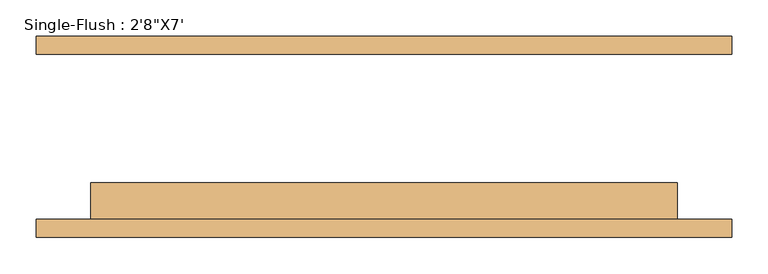
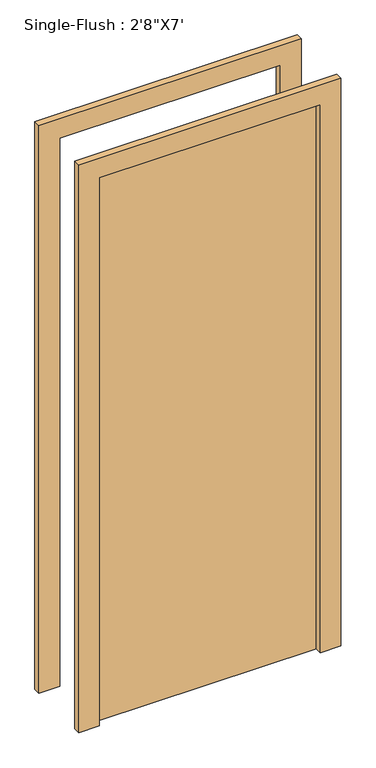
"""IFC4 building model written with IfcOpenShell, lengths in millimetres: door geometry."""

from ifc_helpers import new_model, si_unit, frame, origin, origin_with_axes, place, context, project, spatial, polyline, outline, extrude, source, transform, mapped, element, save


def door_7b345704(model_context):
    return source(origin(), model_context, "Body", "SweptSolid", [
        extrude(outline(polyline([(2209.8, -482.6), (0.0, -482.6), (0.0, -406.4), (2133.6, -406.4), (2133.6, 406.4), (0.0, 406.4), (0.0, 482.6), (2209.8, 482.6), (2209.8, -482.6)])), frame((0.0, -139.7, 0.0), z_axis=(0.0, 1.0, 0.0), x_axis=(0.0, 0.0, 1.0)), (0.0, 0.0, 1.0), 25.4),
        extrude(outline(polyline([(2209.8, 482.6), (2209.8, -482.6), (0.0, -482.6), (0.0, -406.4), (2133.6, -406.4), (2133.6, 406.4), (0.0, 406.4), (0.0, 482.6), (2209.8, 482.6)])), frame((0.0, 114.3, 0.0), z_axis=(0.0, 1.0, 0.0), x_axis=(0.0, 0.0, 1.0)), (0.0, 0.0, 1.0), 25.4),
        extrude(outline(polyline([(406.4, -63.5), (406.4, -114.3), (-406.4, -114.3), (-406.4, -63.5), (406.4, -63.5)])), origin_with_axes(), (0.0, 0.0, 1.0), 2133.6),
    ])


if __name__ == "__main__":
    model = new_model("IFC4")
    model_context = context("Model", 3, world=origin())
    ifc_project = project(units=[si_unit("LENGTHUNIT", "METRE", prefix="MILLI")], contexts=[model_context])
    site = spatial("IfcSite", under=ifc_project)
    building = spatial("IfcBuilding", under=site)
    placement = place(None, origin())
    door_shape = door_7b345704(model_context)
    element("IfcDoor", 1, ObjectType="Single-Flush : 2'8\"X7'", at=placement, inside=building, context=model_context, shape_type="MappedRepresentation", body=[
        mapped(door_shape, transform((0.0, 0.0, 0.0), x_axis=(1.0, 0.0, 0.0), y_axis=(0.0, 1.0, 0.0), z_axis=(0.0, 0.0, 1.0))),
    ])
    save(model, "model.ifc")

# Revit data of these elements
# Type "Single-Flush : 2'8\"X7'"
#   Type Mark = "9"
#   Construction Type Id = "MDOOR"
#   Assembly Code = "C1020"
#   Analytic Construction = "Metal"
#   Thickness = 0' - 2"
#   Heat Transfer Coefficient (U) = 0.651978 BTU/(h·ft²·°F)
#   Height = 7' - 0"
#   Trim Projection Ext = 0' - 1"
#   Trim Projection Int = 0' - 1"
#   Trim Width = 0' - 3"
#   Width = 2' - 8"
#   Define Thermal Properties by = 1
#   Door Material = Door - Panel
#   Frame Material = Door - Frame
#   Visual Light Transmittance = 0
#   Solar Heat Gain Coefficient = 0
#   Function = (empty or 0)
#   Wall Closure = (empty or 0)
# Element 1 (IfcDoor, "Single-Flush : 2'8\"X7'")
#   Materials on its faces: "Door - Frame", "Door - Panel"
# Materials
#   "Door - Panel": class "Wood", colour RGB 210 159 95, transparency 0, Cost = 0
#   "Door - Frame": colour RGB 118 70 51, transparency 0, Cost = 0
